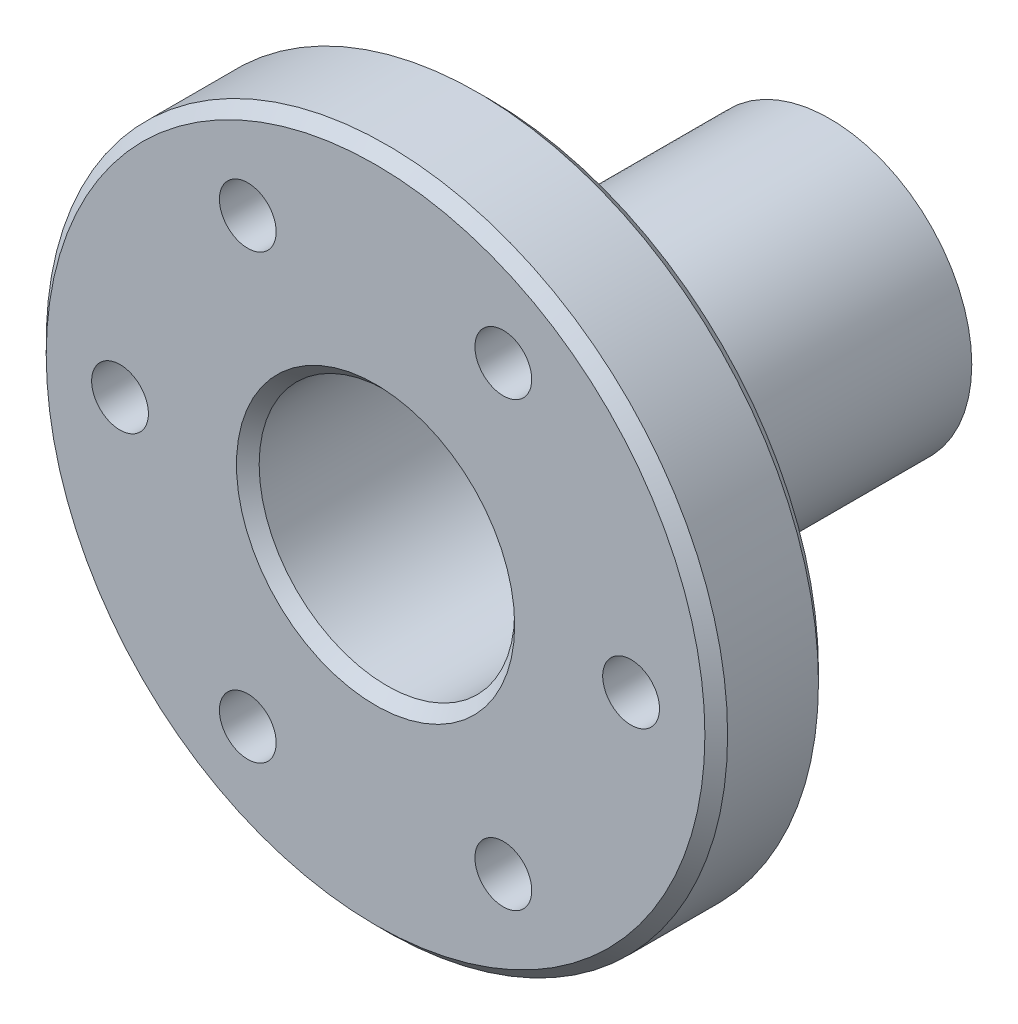
ISO-10303-21;
HEADER;
FILE_DESCRIPTION(('STEP AP214'),'2;1');
FILE_NAME('part.step','',(''),(''),'','','');
FILE_SCHEMA(('AUTOMOTIVE_DESIGN { 1 0 10303 214 1 1 1 1 }'));
ENDSEC;
DATA;
#1=APPLICATION_CONTEXT('core data for automotive mechanical design processes');
#2=APPLICATION_PROTOCOL_DEFINITION('international standard','automotive_design',2000,#1);
#3=PRODUCT_CONTEXT('',#1,'mechanical');
#4=PRODUCT('Part','Part','',(#3));
#5=PRODUCT_RELATED_PRODUCT_CATEGORY('part','',(#4));
#6=PRODUCT_DEFINITION_FORMATION('','',#4);
#7=PRODUCT_DEFINITION_CONTEXT('part definition',#1,'design');
#8=PRODUCT_DEFINITION('design','',#6,#7);
#9=PRODUCT_DEFINITION_SHAPE('','',#8);
#10=(LENGTH_UNIT() NAMED_UNIT(*) SI_UNIT(.MILLI.,.METRE.));
#11=(NAMED_UNIT(*) PLANE_ANGLE_UNIT() SI_UNIT($,.RADIAN.));
#12=(NAMED_UNIT(*) SI_UNIT($,.STERADIAN.) SOLID_ANGLE_UNIT());
#13=UNCERTAINTY_MEASURE_WITH_UNIT(LENGTH_MEASURE(1.E-05),#10,'distance_accuracy_value','');
#14=(GEOMETRIC_REPRESENTATION_CONTEXT(3) GLOBAL_UNCERTAINTY_ASSIGNED_CONTEXT((#13)) GLOBAL_UNIT_ASSIGNED_CONTEXT((#10,
#11,#12)) REPRESENTATION_CONTEXT('',''));
#15=CARTESIAN_POINT('',(0.,0.,0.));
#16=DIRECTION('',(0.,0.,1.));
#17=DIRECTION('',(1.,0.,0.));
#18=AXIS2_PLACEMENT_3D('',#15,#16,#17);
#19=CARTESIAN_POINT('',(0.,0.,20.));
#20=DIRECTION('',(0.,0.,1.));
#21=DIRECTION('',(1.,0.,0.));
#22=AXIS2_PLACEMENT_3D('',#19,#20,#21);
#23=PLANE('',#22);
#24=CARTESIAN_POINT('',(0.,0.,20.));
#25=DIRECTION('',(0.,0.,1.));
#26=DIRECTION('',(1.,0.,0.));
#27=AXIS2_PLACEMENT_3D('',#24,#25,#26);
#28=CIRCLE('',#27,58.);
#29=CARTESIAN_POINT('',(58.,0.,20.));
#30=VERTEX_POINT('',#29);
#31=EDGE_CURVE('E10',#30,#30,#28,.T.);
#32=ORIENTED_EDGE('',*,*,#31,.T.);
#33=EDGE_LOOP('',(#32));
#34=FACE_BOUND('',#33,.T.);
#35=CARTESIAN_POINT('',(0.,0.,20.));
#36=DIRECTION('',(0.,0.,1.));
#37=DIRECTION('',(1.,0.,0.));
#38=AXIS2_PLACEMENT_3D('',#35,#36,#37);
#39=CIRCLE('',#38,24.5);
#40=CARTESIAN_POINT('',(24.5,0.,20.));
#41=VERTEX_POINT('',#40);
#42=EDGE_CURVE('E50',#41,#41,#39,.F.);
#43=ORIENTED_EDGE('',*,*,#42,.T.);
#44=EDGE_LOOP('',(#43));
#45=FACE_BOUND('',#44,.T.);
#46=CARTESIAN_POINT('',(-22.4999999999996,38.9711431703,20.));
#47=DIRECTION('',(0.,0.,1.));
#48=DIRECTION('',(1.,0.,0.));
#49=AXIS2_PLACEMENT_3D('',#46,#47,#48);
#50=CIRCLE('',#49,4.99999999999999);
#51=CARTESIAN_POINT('',(-17.4999999999997,38.9711431703,20.));
#52=VERTEX_POINT('',#51);
#53=EDGE_CURVE('E99',#52,#52,#50,.T.);
#54=ORIENTED_EDGE('',*,*,#53,.F.);
#55=EDGE_LOOP('',(#54));
#56=FACE_BOUND('',#55,.T.);
#57=CARTESIAN_POINT('',(-22.5000000000002,-38.9711431702996,20.));
#58=DIRECTION('',(0.,0.,1.));
#59=DIRECTION('',(1.,0.,0.));
#60=AXIS2_PLACEMENT_3D('',#57,#58,#59);
#61=CIRCLE('',#60,5.);
#62=CARTESIAN_POINT('',(-17.5000000000002,-38.9711431702996,20.));
#63=VERTEX_POINT('',#62);
#64=EDGE_CURVE('E86',#63,#63,#61,.T.);
#65=ORIENTED_EDGE('',*,*,#64,.F.);
#66=EDGE_LOOP('',(#65));
#67=FACE_BOUND('',#66,.T.);
#68=CARTESIAN_POINT('',(45.,0.,20.));
#69=DIRECTION('',(0.,0.,1.));
#70=DIRECTION('',(1.,0.,0.));
#71=AXIS2_PLACEMENT_3D('',#68,#69,#70);
#72=CIRCLE('',#71,5.);
#73=CARTESIAN_POINT('',(50.,0.,20.));
#74=VERTEX_POINT('',#73);
#75=EDGE_CURVE('E76',#74,#74,#72,.T.);
#76=ORIENTED_EDGE('',*,*,#75,.F.);
#77=EDGE_LOOP('',(#76));
#78=FACE_BOUND('',#77,.T.);
#79=CARTESIAN_POINT('',(22.5,-38.9711431702991,20.));
#80=DIRECTION('',(0.,0.,1.));
#81=DIRECTION('',(1.,0.,0.));
#82=AXIS2_PLACEMENT_3D('',#79,#80,#81);
#83=CIRCLE('',#82,5.00000000000042);
#84=CARTESIAN_POINT('',(27.5000000000004,-38.9711431702991,20.));
#85=VERTEX_POINT('',#84);
#86=EDGE_CURVE('E85',#85,#85,#83,.T.);
#87=ORIENTED_EDGE('',*,*,#86,.F.);
#88=EDGE_LOOP('',(#87));
#89=FACE_BOUND('',#88,.T.);
#90=CARTESIAN_POINT('',(-45.,3.14233320495882E-13,20.));
#91=DIRECTION('',(0.,0.,1.));
#92=DIRECTION('',(1.,0.,0.));
#93=AXIS2_PLACEMENT_3D('',#90,#91,#92);
#94=CIRCLE('',#93,4.99999999999999);
#95=CARTESIAN_POINT('',(-40.,3.14233320495882E-13,20.));
#96=VERTEX_POINT('',#95);
#97=EDGE_CURVE('E92',#96,#96,#94,.T.);
#98=ORIENTED_EDGE('',*,*,#97,.F.);
#99=EDGE_LOOP('',(#98));
#100=FACE_BOUND('',#99,.T.);
#101=CARTESIAN_POINT('',(22.5000000000005,38.9711431702995,20.));
#102=DIRECTION('',(0.,0.,1.));
#103=DIRECTION('',(1.,0.,0.));
#104=AXIS2_PLACEMENT_3D('',#101,#102,#103);
#105=CIRCLE('',#104,5.);
#106=CARTESIAN_POINT('',(27.5000000000005,38.9711431702995,20.));
#107=VERTEX_POINT('',#106);
#108=EDGE_CURVE('E106',#107,#107,#105,.T.);
#109=ORIENTED_EDGE('',*,*,#108,.F.);
#110=EDGE_LOOP('',(#109));
#111=FACE_BOUND('',#110,.T.);
#112=ADVANCED_FACE('F39',(#34,#45,#56,#67,#78,#89,#100,#111),#23,.T.);
#113=CARTESIAN_POINT('',(0.,0.,0.));
#114=DIRECTION('',(0.,0.,1.));
#115=DIRECTION('',(1.,0.,0.));
#116=AXIS2_PLACEMENT_3D('',#113,#114,#115);
#117=PLANE('',#116);
#118=CARTESIAN_POINT('',(0.,0.,0.));
#119=DIRECTION('',(0.,0.,1.));
#120=DIRECTION('',(1.,0.,0.));
#121=AXIS2_PLACEMENT_3D('',#118,#119,#120);
#122=CIRCLE('',#121,58.);
#123=CARTESIAN_POINT('',(58.,0.,0.));
#124=VERTEX_POINT('',#123);
#125=EDGE_CURVE('E64',#124,#124,#122,.F.);
#126=ORIENTED_EDGE('',*,*,#125,.T.);
#127=EDGE_LOOP('',(#126));
#128=FACE_BOUND('',#127,.T.);
#129=CARTESIAN_POINT('',(0.,0.,0.));
#130=DIRECTION('',(0.,0.,1.));
#131=DIRECTION('',(1.,0.,0.));
#132=AXIS2_PLACEMENT_3D('',#129,#130,#131);
#133=CIRCLE('',#132,28.);
#134=CARTESIAN_POINT('',(28.,0.,0.));
#135=VERTEX_POINT('',#134);
#136=EDGE_CURVE('E75',#135,#135,#133,.T.);
#137=ORIENTED_EDGE('',*,*,#136,.T.);
#138=EDGE_LOOP('',(#137));
#139=FACE_BOUND('',#138,.T.);
#140=CARTESIAN_POINT('',(45.,0.,0.));
#141=DIRECTION('',(0.,0.,1.));
#142=DIRECTION('',(1.,0.,0.));
#143=AXIS2_PLACEMENT_3D('',#140,#141,#142);
#144=CIRCLE('',#143,5.);
#145=CARTESIAN_POINT('',(50.,0.,0.));
#146=VERTEX_POINT('',#145);
#147=EDGE_CURVE('E79',#146,#146,#144,.T.);
#148=ORIENTED_EDGE('',*,*,#147,.T.);
#149=EDGE_LOOP('',(#148));
#150=FACE_BOUND('',#149,.T.);
#151=CARTESIAN_POINT('',(22.5,-38.9711431702991,0.));
#152=DIRECTION('',(0.,0.,1.));
#153=DIRECTION('',(1.,0.,0.));
#154=AXIS2_PLACEMENT_3D('',#151,#152,#153);
#155=CIRCLE('',#154,5.00000000000042);
#156=CARTESIAN_POINT('',(27.5000000000004,-38.9711431702991,0.));
#157=VERTEX_POINT('',#156);
#158=EDGE_CURVE('E83',#157,#157,#155,.T.);
#159=ORIENTED_EDGE('',*,*,#158,.T.);
#160=EDGE_LOOP('',(#159));
#161=FACE_BOUND('',#160,.T.);
#162=CARTESIAN_POINT('',(-22.5000000000002,-38.9711431702996,0.));
#163=DIRECTION('',(0.,0.,1.));
#164=DIRECTION('',(1.,0.,0.));
#165=AXIS2_PLACEMENT_3D('',#162,#163,#164);
#166=CIRCLE('',#165,5.);
#167=CARTESIAN_POINT('',(-17.5000000000002,-38.9711431702996,0.));
#168=VERTEX_POINT('',#167);
#169=EDGE_CURVE('E93',#168,#168,#166,.T.);
#170=ORIENTED_EDGE('',*,*,#169,.T.);
#171=EDGE_LOOP('',(#170));
#172=FACE_BOUND('',#171,.T.);
#173=CARTESIAN_POINT('',(-45.,3.14233320495882E-13,0.));
#174=DIRECTION('',(0.,0.,1.));
#175=DIRECTION('',(1.,0.,0.));
#176=AXIS2_PLACEMENT_3D('',#173,#174,#175);
#177=CIRCLE('',#176,4.99999999999999);
#178=CARTESIAN_POINT('',(-40.,3.14233320495882E-13,0.));
#179=VERTEX_POINT('',#178);
#180=EDGE_CURVE('E97',#179,#179,#177,.T.);
#181=ORIENTED_EDGE('',*,*,#180,.T.);
#182=EDGE_LOOP('',(#181));
#183=FACE_BOUND('',#182,.T.);
#184=CARTESIAN_POINT('',(-22.4999999999996,38.9711431703,0.));
#185=DIRECTION('',(0.,0.,1.));
#186=DIRECTION('',(1.,0.,0.));
#187=AXIS2_PLACEMENT_3D('',#184,#185,#186);
#188=CIRCLE('',#187,4.99999999999999);
#189=CARTESIAN_POINT('',(-17.4999999999997,38.9711431703,0.));
#190=VERTEX_POINT('',#189);
#191=EDGE_CURVE('E101',#190,#190,#188,.T.);
#192=ORIENTED_EDGE('',*,*,#191,.T.);
#193=EDGE_LOOP('',(#192));
#194=FACE_BOUND('',#193,.T.);
#195=CARTESIAN_POINT('',(22.5000000000005,38.9711431702995,0.));
#196=DIRECTION('',(0.,0.,1.));
#197=DIRECTION('',(1.,0.,0.));
#198=AXIS2_PLACEMENT_3D('',#195,#196,#197);
#199=CIRCLE('',#198,5.);
#200=CARTESIAN_POINT('',(27.5000000000005,38.9711431702995,0.));
#201=VERTEX_POINT('',#200);
#202=EDGE_CURVE('E107',#201,#201,#199,.T.);
#203=ORIENTED_EDGE('',*,*,#202,.T.);
#204=EDGE_LOOP('',(#203));
#205=FACE_BOUND('',#204,.T.);
#206=ADVANCED_FACE('F140',(#128,#139,#150,#161,#172,#183,#194,#205),#117,.F.);
#207=CARTESIAN_POINT('',(0.,0.,20.));
#208=DIRECTION('',(0.,0.,-1.));
#209=DIRECTION('',(-1.,0.,0.));
#210=AXIS2_PLACEMENT_3D('',#207,#208,#209);
#211=CYLINDRICAL_SURFACE('',#210,60.);
#212=CARTESIAN_POINT('',(0.,0.,2.00000000000001));
#213=DIRECTION('',(0.,0.,1.));
#214=DIRECTION('',(1.,0.,0.));
#215=AXIS2_PLACEMENT_3D('',#212,#213,#214);
#216=CIRCLE('',#215,60.);
#217=CARTESIAN_POINT('',(60.,0.,2.00000000000001));
#218=VERTEX_POINT('',#217);
#219=EDGE_CURVE('E68',#218,#218,#216,.T.);
#220=ORIENTED_EDGE('',*,*,#219,.T.);
#221=EDGE_LOOP('',(#220));
#222=FACE_BOUND('',#221,.T.);
#223=CARTESIAN_POINT('',(0.,0.,18.));
#224=DIRECTION('',(0.,0.,1.));
#225=DIRECTION('',(1.,0.,0.));
#226=AXIS2_PLACEMENT_3D('',#223,#224,#225);
#227=CIRCLE('',#226,60.);
#228=CARTESIAN_POINT('',(60.,0.,18.));
#229=VERTEX_POINT('',#228);
#230=EDGE_CURVE('E67',#229,#229,#227,.F.);
#231=ORIENTED_EDGE('',*,*,#230,.T.);
#232=EDGE_LOOP('',(#231));
#233=FACE_BOUND('',#232,.T.);
#234=ADVANCED_FACE('F145',(#222,#233),#211,.T.);
#235=CARTESIAN_POINT('',(0.,0.,20.));
#236=DIRECTION('',(0.,0.,-1.));
#237=DIRECTION('',(-1.,0.,0.));
#238=AXIS2_PLACEMENT_3D('',#235,#236,#237);
#239=CYLINDRICAL_SURFACE('',#238,22.5);
#240=CARTESIAN_POINT('',(0.,0.,-58.));
#241=DIRECTION('',(0.,0.,-1.));
#242=DIRECTION('',(-1.,0.,0.));
#243=AXIS2_PLACEMENT_3D('',#240,#241,#242);
#244=CIRCLE('',#243,22.5);
#245=CARTESIAN_POINT('',(-22.5,0.,-58.));
#246=VERTEX_POINT('',#245);
#247=EDGE_CURVE('E54',#246,#246,#244,.T.);
#248=ORIENTED_EDGE('',*,*,#247,.T.);
#249=EDGE_LOOP('',(#248));
#250=FACE_BOUND('',#249,.T.);
#251=CARTESIAN_POINT('',(0.,0.,18.));
#252=DIRECTION('',(0.,0.,1.));
#253=DIRECTION('',(1.,0.,0.));
#254=AXIS2_PLACEMENT_3D('',#251,#252,#253);
#255=CIRCLE('',#254,22.5);
#256=CARTESIAN_POINT('',(22.5,0.,18.));
#257=VERTEX_POINT('',#256);
#258=EDGE_CURVE('E58',#257,#257,#255,.T.);
#259=ORIENTED_EDGE('',*,*,#258,.T.);
#260=EDGE_LOOP('',(#259));
#261=FACE_BOUND('',#260,.T.);
#262=ADVANCED_FACE('F147',(#250,#261),#239,.F.);
#263=CARTESIAN_POINT('',(45.,0.,20.));
#264=DIRECTION('',(0.,0.,-1.));
#265=DIRECTION('',(-1.,0.,0.));
#266=AXIS2_PLACEMENT_3D('',#263,#264,#265);
#267=CYLINDRICAL_SURFACE('',#266,5.);
#268=ORIENTED_EDGE('',*,*,#75,.T.);
#269=EDGE_LOOP('',(#268));
#270=FACE_BOUND('',#269,.T.);
#271=ORIENTED_EDGE('',*,*,#147,.F.);
#272=EDGE_LOOP('',(#271));
#273=FACE_BOUND('',#272,.T.);
#274=ADVANCED_FACE('F187',(#270,#273),#267,.F.);
#275=CARTESIAN_POINT('',(22.5,-38.9711431702991,20.));
#276=DIRECTION('',(0.,0.,-1.));
#277=DIRECTION('',(-1.,0.,0.));
#278=AXIS2_PLACEMENT_3D('',#275,#276,#277);
#279=CYLINDRICAL_SURFACE('',#278,5.00000000000042);
#280=ORIENTED_EDGE('',*,*,#86,.T.);
#281=EDGE_LOOP('',(#280));
#282=FACE_BOUND('',#281,.T.);
#283=ORIENTED_EDGE('',*,*,#158,.F.);
#284=EDGE_LOOP('',(#283));
#285=FACE_BOUND('',#284,.T.);
#286=ADVANCED_FACE('F192',(#282,#285),#279,.F.);
#287=CARTESIAN_POINT('',(-22.5000000000002,-38.9711431702996,20.));
#288=DIRECTION('',(0.,0.,-1.));
#289=DIRECTION('',(-1.,0.,0.));
#290=AXIS2_PLACEMENT_3D('',#287,#288,#289);
#291=CYLINDRICAL_SURFACE('',#290,5.);
#292=ORIENTED_EDGE('',*,*,#64,.T.);
#293=EDGE_LOOP('',(#292));
#294=FACE_BOUND('',#293,.T.);
#295=ORIENTED_EDGE('',*,*,#169,.F.);
#296=EDGE_LOOP('',(#295));
#297=FACE_BOUND('',#296,.T.);
#298=ADVANCED_FACE('F196',(#294,#297),#291,.F.);
#299=CARTESIAN_POINT('',(-45.,3.14233320495882E-13,20.));
#300=DIRECTION('',(0.,0.,-1.));
#301=DIRECTION('',(-1.,0.,0.));
#302=AXIS2_PLACEMENT_3D('',#299,#300,#301);
#303=CYLINDRICAL_SURFACE('',#302,4.99999999999999);
#304=ORIENTED_EDGE('',*,*,#97,.T.);
#305=EDGE_LOOP('',(#304));
#306=FACE_BOUND('',#305,.T.);
#307=ORIENTED_EDGE('',*,*,#180,.F.);
#308=EDGE_LOOP('',(#307));
#309=FACE_BOUND('',#308,.T.);
#310=ADVANCED_FACE('F204',(#306,#309),#303,.F.);
#311=CARTESIAN_POINT('',(-22.4999999999996,38.9711431703,20.));
#312=DIRECTION('',(0.,0.,-1.));
#313=DIRECTION('',(-1.,0.,0.));
#314=AXIS2_PLACEMENT_3D('',#311,#312,#313);
#315=CYLINDRICAL_SURFACE('',#314,4.99999999999999);
#316=ORIENTED_EDGE('',*,*,#53,.T.);
#317=EDGE_LOOP('',(#316));
#318=FACE_BOUND('',#317,.T.);
#319=ORIENTED_EDGE('',*,*,#191,.F.);
#320=EDGE_LOOP('',(#319));
#321=FACE_BOUND('',#320,.T.);
#322=ADVANCED_FACE('F131',(#318,#321),#315,.F.);
#323=CARTESIAN_POINT('',(22.5000000000005,38.9711431702995,20.));
#324=DIRECTION('',(0.,0.,-1.));
#325=DIRECTION('',(-1.,0.,0.));
#326=AXIS2_PLACEMENT_3D('',#323,#324,#325);
#327=CYLINDRICAL_SURFACE('',#326,5.);
#328=ORIENTED_EDGE('',*,*,#108,.T.);
#329=EDGE_LOOP('',(#328));
#330=FACE_BOUND('',#329,.T.);
#331=ORIENTED_EDGE('',*,*,#202,.F.);
#332=EDGE_LOOP('',(#331));
#333=FACE_BOUND('',#332,.T.);
#334=ADVANCED_FACE('F125',(#330,#333),#327,.F.);
#335=CARTESIAN_POINT('',(0.,0.,-60.));
#336=DIRECTION('',(0.,0.,1.));
#337=DIRECTION('',(1.,0.,0.));
#338=AXIS2_PLACEMENT_3D('',#335,#336,#337);
#339=CYLINDRICAL_SURFACE('',#338,25.);
#340=CARTESIAN_POINT('',(0.,0.,-3.));
#341=DIRECTION('',(0.,0.,1.));
#342=DIRECTION('',(1.,0.,0.));
#343=AXIS2_PLACEMENT_3D('',#340,#341,#342);
#344=CIRCLE('',#343,25.);
#345=CARTESIAN_POINT('',(25.,0.,-3.));
#346=VERTEX_POINT('',#345);
#347=EDGE_CURVE('E74',#346,#346,#344,.F.);
#348=ORIENTED_EDGE('',*,*,#347,.T.);
#349=EDGE_LOOP('',(#348));
#350=FACE_BOUND('',#349,.T.);
#351=CARTESIAN_POINT('',(0.,0.,-60.));
#352=DIRECTION('',(0.,0.,-1.));
#353=DIRECTION('',(-1.,0.,0.));
#354=AXIS2_PLACEMENT_3D('',#351,#352,#353);
#355=CIRCLE('',#354,25.);
#356=CARTESIAN_POINT('',(-25.,0.,-60.));
#357=VERTEX_POINT('',#356);
#358=EDGE_CURVE('E115',#357,#357,#355,.T.);
#359=ORIENTED_EDGE('',*,*,#358,.F.);
#360=EDGE_LOOP('',(#359));
#361=FACE_BOUND('',#360,.T.);
#362=ADVANCED_FACE('F119',(#350,#361),#339,.T.);
#363=CARTESIAN_POINT('',(0.,0.,-60.));
#364=DIRECTION('',(0.,0.,-1.));
#365=DIRECTION('',(-1.,0.,0.));
#366=AXIS2_PLACEMENT_3D('',#363,#364,#365);
#367=PLANE('',#366);
#368=CARTESIAN_POINT('',(0.,0.,-60.));
#369=DIRECTION('',(0.,0.,-1.));
#370=DIRECTION('',(-1.,0.,0.));
#371=AXIS2_PLACEMENT_3D('',#368,#369,#370);
#372=CIRCLE('',#371,24.5);
#373=CARTESIAN_POINT('',(-24.5,0.,-60.));
#374=VERTEX_POINT('',#373);
#375=EDGE_CURVE('E51',#374,#374,#372,.F.);
#376=ORIENTED_EDGE('',*,*,#375,.T.);
#377=EDGE_LOOP('',(#376));
#378=FACE_BOUND('',#377,.T.);
#379=ORIENTED_EDGE('',*,*,#358,.T.);
#380=EDGE_LOOP('',(#379));
#381=FACE_BOUND('',#380,.T.);
#382=ADVANCED_FACE('F117',(#378,#381),#367,.T.);
#383=CARTESIAN_POINT('',(0.,0.,-3.));
#384=DIRECTION('',(0.,0.,1.));
#385=DIRECTION('',(1.,0.,0.));
#386=AXIS2_PLACEMENT_3D('',#383,#384,#385);
#387=TOROIDAL_SURFACE('',#386,28.,3.);
#388=ORIENTED_EDGE('',*,*,#136,.F.);
#389=EDGE_LOOP('',(#388));
#390=FACE_BOUND('',#389,.T.);
#391=ORIENTED_EDGE('',*,*,#347,.F.);
#392=EDGE_LOOP('',(#391));
#393=FACE_BOUND('',#392,.T.);
#394=ADVANCED_FACE('F128',(#390,#393),#387,.F.);
#395=CARTESIAN_POINT('',(0.,0.,2.00000000000001));
#396=DIRECTION('',(0.,0.,1.));
#397=DIRECTION('',(1.,0.,0.));
#398=AXIS2_PLACEMENT_3D('',#395,#396,#397);
#399=CONICAL_SURFACE('',#398,60.,0.785398163397445);
#400=ORIENTED_EDGE('',*,*,#125,.F.);
#401=EDGE_LOOP('',(#400));
#402=FACE_BOUND('',#401,.T.);
#403=ORIENTED_EDGE('',*,*,#219,.F.);
#404=EDGE_LOOP('',(#403));
#405=FACE_BOUND('',#404,.T.);
#406=ADVANCED_FACE('F151',(#402,#405),#399,.T.);
#407=CARTESIAN_POINT('',(0.,0.,-58.));
#408=DIRECTION('',(0.,0.,-1.));
#409=DIRECTION('',(-1.,0.,0.));
#410=AXIS2_PLACEMENT_3D('',#407,#408,#409);
#411=CONICAL_SURFACE('',#410,22.5,0.785398163397455);
#412=ORIENTED_EDGE('',*,*,#375,.F.);
#413=EDGE_LOOP('',(#412));
#414=FACE_BOUND('',#413,.T.);
#415=ORIENTED_EDGE('',*,*,#247,.F.);
#416=EDGE_LOOP('',(#415));
#417=FACE_BOUND('',#416,.T.);
#418=ADVANCED_FACE('F163',(#414,#417),#411,.F.);
#419=CARTESIAN_POINT('',(0.,0.,20.));
#420=DIRECTION('',(0.,0.,-1.));
#421=DIRECTION('',(-1.,0.,0.));
#422=AXIS2_PLACEMENT_3D('',#419,#420,#421);
#423=CONICAL_SURFACE('',#422,58.,0.785398163397453);
#424=ORIENTED_EDGE('',*,*,#230,.F.);
#425=EDGE_LOOP('',(#424));
#426=FACE_BOUND('',#425,.T.);
#427=ORIENTED_EDGE('',*,*,#31,.F.);
#428=EDGE_LOOP('',(#427));
#429=FACE_BOUND('',#428,.T.);
#430=ADVANCED_FACE('F170',(#426,#429),#423,.T.);
#431=CARTESIAN_POINT('',(0.,0.,18.));
#432=DIRECTION('',(0.,0.,1.));
#433=DIRECTION('',(1.,0.,0.));
#434=AXIS2_PLACEMENT_3D('',#431,#432,#433);
#435=CONICAL_SURFACE('',#434,22.5,0.785398163397455);
#436=ORIENTED_EDGE('',*,*,#42,.F.);
#437=EDGE_LOOP('',(#436));
#438=FACE_BOUND('',#437,.T.);
#439=ORIENTED_EDGE('',*,*,#258,.F.);
#440=EDGE_LOOP('',(#439));
#441=FACE_BOUND('',#440,.T.);
#442=ADVANCED_FACE('F45',(#438,#441),#435,.F.);
#443=CLOSED_SHELL('',(#112,#206,#234,#262,#274,#286,#298,#310,#322,#334,#362,#382,#394,#406,
#418,#430,#442));
#444=MANIFOLD_SOLID_BREP('B2',#443);
#445=ADVANCED_BREP_SHAPE_REPRESENTATION('',(#18,#444),#14);
#446=SHAPE_DEFINITION_REPRESENTATION(#9,#445);
ENDSEC;
END-ISO-10303-21;
